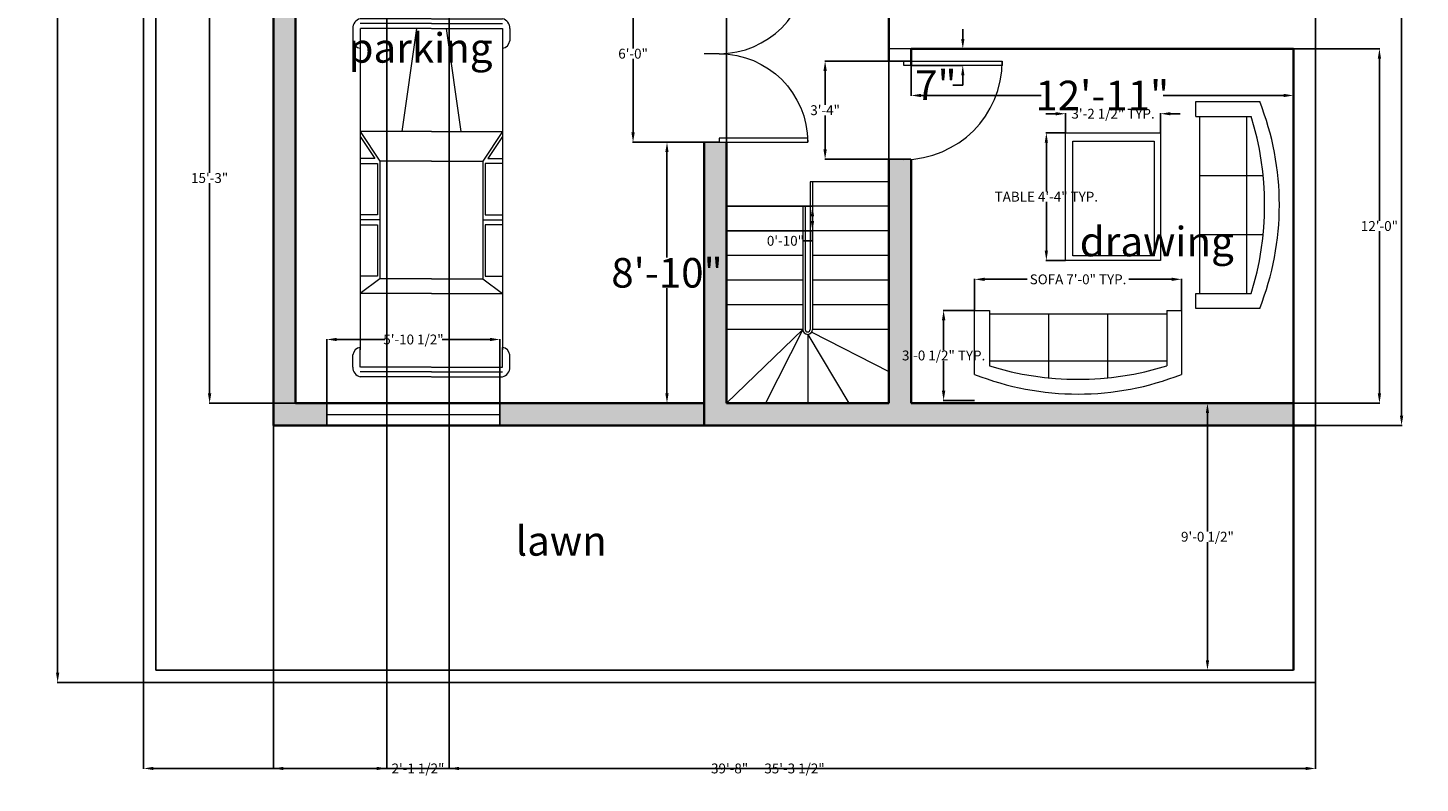
# Model space of a CAD drawing. Units: inches. Extents: x -346 to 220, y 97 to 877.
# Tile 1 of 4: x -346 to 220, y 97 to 404. Entities that reach past the tile are written whole.
import ezdxf

# ---------------------------------------------------------------- set-up
doc = ezdxf.new("R2010")
doc.units = ezdxf.units.IN
doc.header["$MEASUREMENT"] = 0
doc.layers.get('0').update_dxf_attribs({"color": 3})
for name, color, linetype, lineweight in [('A-AREA-IDEN', 130, 'Continuous', 25), ('A-FLOR-STRS', 3, 'Continuous', 18), ('A-FURN', 8, 'Continuous', 18), ('A-WALL', 7, 'Continuous', 35), ('C-PRKG-VEHI', 8, 'Continuous', 13), ('C-PROP', 94, 'Continuous', 25), ('dim', 170, 'Continuous', 13), ('door', 20, 'Continuous', 18)]:
    doc.layers.add(name, color=color, linetype=linetype, lineweight=lineweight)
doc.layers.add('A-WALL-PATT', color=61, linetype='Continuous', lineweight=13, true_color=0xe5e878)
doc.styles.get("Standard").update_dxf_attribs({"font": 'arial.ttf'})
doc.dimstyles.get("Standard").update_dxf_attribs({"dimtxt": 4, "dimasz": 4, "dimexe": 0.18, "dimexo": 0.0625, "dimgap": 0.09, "dimtad": 0, "dimtih": 1, "dimtoh": 1, "dimdec": 0, "dimzin": 0, "dimdsep": 46, "dimlunit": 3, "dimtxsty": 'Standard', "dimcen": 0.09, "dimadec": 0, "dimazin": 0, "dimtfac": 1, "dimtdec": 0, "dimtofl": 0, "dimtmove": 0, "dimatfit": 3, "dimfxl": 1, "dimtolj": 1, "dimtzin": 0, "dimarcsym": 0})

# ---------------------------------------------------------------- blocks, each defined once
blk = doc.blocks.new('*D7')
at = {"layer": 'Defpoints', "color": 0, "transparency": 16777216}
for p in [(-71.23, 357.75), (-86.38, 251.75), (-71.23, 251.75)]:
    blk.add_point(p, dxfattribs=at)
at = {"layer": 'dim', "color": 0, "lineweight": -2, "transparency": 16777216}
for p, q in [((-71.29, 357.75), (-86.56, 357.75)), ((-86.38, 353.75), (-86.38, 310.96)), ((-86.38, 255.75), (-86.38, 298.53)), ((-71.29, 251.75), (-86.56, 251.75))]:
    blk.add_line(p, q, dxfattribs=at)
at = {"layer": 'dim', "color": 0, "transparency": 16777216}
for points in [[(-87.05, 353.75), (-85.72, 353.75), (-86.38, 357.75)], [(-87.05, 255.75), (-85.72, 255.75), (-86.38, 251.75)]]:
    blk.add_solid(points, dxfattribs=at)
at = {"layer": 'dim', "color": 0, "transparency": 16777216, "insert": (-86.38, 304.75), "char_height": 4, "attachment_point": 5}
blk.add_mtext('\\A1;{\\H3x;8\'-10"}', dxfattribs=at)
blk = doc.blocks.new('*D9')
at = {"layer": 'Defpoints', "color": 0, "transparency": 16777216}
for p in [(12.77, 395.75), (168.07, 395.75), (168.07, 376.78)]:
    blk.add_point(p, dxfattribs=at)
at = {"layer": 'dim', "color": 0, "lineweight": -2, "transparency": 16777216}
for p, q in [((12.77, 395.68), (12.77, 376.6)), ((168.07, 395.68), (168.07, 376.6)), ((16.77, 376.78), (65.62, 376.78)), ((164.07, 376.78), (115.22, 376.78))]:
    blk.add_line(p, q, dxfattribs=at)
at = {"layer": 'dim', "color": 0, "transparency": 16777216}
for points in [[(16.77, 377.44), (16.77, 376.11), (12.77, 376.78)], [(164.07, 377.44), (164.07, 376.11), (168.07, 376.78)]]:
    blk.add_solid(points, dxfattribs=at)
at = {"layer": 'dim', "color": 0, "transparency": 16777216, "insert": (90.42, 376.78), "char_height": 4, "attachment_point": 5}
blk.add_mtext('\\A1;{\\H3x;12\'-11"}', dxfattribs=at)
blk = doc.blocks.new('*D10')
at = {"layer": 'Defpoints', "color": 0, "transparency": 16777216}
for p in [(12.77, 395.75), (12.77, 389), (33.77, 389)]:
    blk.add_point(p, dxfattribs=at)
at = {"layer": 'dim', "color": 0, "lineweight": -2, "transparency": 16777216}
for p, q in [((33.77, 399.75), (33.77, 403.75)), ((12.84, 395.75), (33.95, 395.75)), ((12.84, 389), (33.95, 389)), ((33.77, 385), (33.77, 381)), ((33.77, 381), (29.77, 381))]:
    blk.add_line(p, q, dxfattribs=at)
at = {"layer": 'dim', "color": 0, "transparency": 16777216}
for points in [[(33.11, 399.75), (34.44, 399.75), (33.77, 395.75)], [(33.11, 385), (34.44, 385), (33.77, 389)]]:
    blk.add_solid(points, dxfattribs=at)
at = {"layer": 'dim', "color": 0, "transparency": 16777216, "insert": (22.84, 381), "char_height": 4, "attachment_point": 5}
blk.add_mtext('\\A1;{\\H3x;7"}', dxfattribs=at)
blk = doc.blocks.new('*U12')
for p, q in [((0, 0), (0, -6)), ((40, 0), (40, -6))]:
    blk.add_line(p, q)
blk.add_lwpolyline([(0, 0), (0, 40), (1.75, 40), (1.75, 0)], close=True)
blk.add_arc((0, 0), 40, 0, 90)
blk = doc.blocks.new('*U13')
for p, q in [((0, 0), (0, -6)), ((36, 0), (36, -6))]:
    blk.add_line(p, q)
blk.add_lwpolyline([(0, 0), (0, 36), (1.75, 36), (1.75, 0)], close=True)
blk.add_arc((0, 0), 36, 0, 90)
blk = doc.blocks.new('Sofa - Roundback 7 ft.')
for p, q in [((-12.00002, -32.4421), (-12.00003, -6.5971)), ((11.99997, -32.4421), (11.99998, -6.5971)), ((-36.000027, -34), (-36.000027, -11.4696)), ((-35.999844, -13.3819), (35.9998, -13.3819)), ((35.99998, -34), (35.99998, -11.4696)), ((-36.000027, -32.4421), (35.99998, -32.4421))]:
    blk.add_line(p, q)
for points in [[(-36.000027, -34), (-42.000027, -34), (-42.000027, -8)], [(41.99998, -8), (41.99998, -34), (35.99998, -34)]]:
    blk.add_lwpolyline(points)
for centre, radius, start, end in [((0, -114.25), 114.25, 68.43141, 111.5686), ((-0.00001, -127.1968), 121.1968, 72.72033, 107.2797)]:
    blk.add_arc(centre, radius, start, end)
blk = doc.blocks.new('*U27')
for p, q in [((0.1, -0.41), (0.1, 38.35)), ((2.77, -0.41), (2.77, 38.31)), ((5.44, 42.31), (12.12, 42.31)), ((5.44, -0.41), (5.44, 38.24)), ((5.45, 38.31), (16.12, 38.31)), ((16.12, 38.31), (180.34, 38.31)), ((61.52, -0.41), (61.52, 38.31)), ((61.52, 38.31), (77.54, 27.62)), ((64.19, 38.31), (76.2, 30.29)), ((76.2, 30.29), (76.2, 38.31)), ((78.87, 38.31), (78.87, 28.96)), ((106.91, 28.96), (106.91, 38.31)), ((109.58, 27.62), (109.58, 38.31)), ((112.25, 38.31), (112.25, 28.96)), ((140.29, 28.96), (140.29, 38.31)), ((141.62, 27.62), (149.64, 38.31)), ((149.64, -0.41), (149.64, 38.31)), ((189.69, 38.31), (179.01, 38.31)), ((189.69, 42.31), (183.01, 42.31)), ((189.69, -0.41), (189.69, 38.24)), ((192.36, -0.41), (192.36, 38.31)), ((195.03, -0.41), (195.03, 38.35)), ((77.54, 27.62), (141.62, 27.62)), ((77.54, -0.41), (77.54, 27.62)), ((78.87, 28.96), (106.91, 28.96)), ((112.25, 28.96), (140.29, 28.96)), ((141.62, -0.41), (141.62, 27.62)), ((5.44, 7.6), (61.52, 15.61)), ((0.1, -0.42), (0.1, -39.18)), ((2.77, -0.41), (2.77, -39.13)), ((5.44, -0.42), (5.44, -39.07)), ((61.52, -0.41), (61.52, -39.13)), ((77.54, -0.41), (77.54, -28.45)), ((141.62, -0.41), (141.62, -28.45)), ((149.64, -0.41), (149.64, -39.13)), ((189.69, -0.42), (189.69, -39.07)), ((192.36, -0.41), (192.36, -39.13)), ((195.03, -0.42), (195.03, -39.18)), ((5.44, -8.42), (61.52, -16.43)), ((61.52, -39.13), (77.54, -28.45)), ((77.54, -28.45), (141.62, -28.45)), ((78.87, -39.13), (78.87, -29.79)), ((78.87, -29.79), (106.91, -29.79)), ((106.91, -29.79), (106.91, -39.13)), ((109.58, -28.45), (109.58, -39.13)), ((112.25, -29.79), (140.29, -29.79)), ((112.25, -39.13), (112.25, -29.79)), ((140.29, -29.79), (140.29, -39.13)), ((141.62, -28.45), (149.64, -39.13)), ((64.19, -39.13), (76.2, -31.12)), ((76.2, -31.12), (76.2, -39.13)), ((5.44, -43.14), (12.12, -43.14)), ((5.45, -39.13), (16.12, -39.13)), ((16.12, -39.13), (180.34, -39.13)), ((189.69, -39.13), (179.01, -39.13)), ((189.69, -43.14), (183.01, -43.14))]:
    blk.add_line(p, q)
for centre, radius, start, end in [((5.06, 37.26), 5.06, 85.64554, 168.0943), ((11.45, 37.64), 4.72, 8.13011, 81.86996), ((183.68, 37.64), 4.72, 98.13004, 171.8699), ((190.07, 37.26), 5.06, 11.90574, 94.35446), ((5.06, -38.09), 5.06, 191.9057, 274.3545), ((11.45, -38.46), 4.72, 278.13, 351.8699), ((183.68, -38.46), 4.72, 188.1301, 261.87), ((190.07, -38.09), 5.06, 265.6455, 348.0943)]:
    blk.add_arc(centre, radius, start, end)
blk = doc.blocks.new('TABLE-COFFEE-RECT')
for points in [[(0, 51.83), (38.64, 51.83), (38.64, 0), (0, 0)], [(2.97, 48.5), (36.03, 48.5), (36.03, 1.93), (2.97, 1.93)]]:
    blk.add_lwpolyline(points, close=True)
blk = doc.blocks.new('*D32')
at = {"layer": 'Defpoints', "color": 0, "transparency": 16777216}
for p in [(38.59, 302.1), (38.59, 289.5), (122.59, 289.5)]:
    blk.add_point(p, dxfattribs=at)
at = {"layer": 'dim', "color": 0, "lineweight": -2, "transparency": 16777216}
for p, q in [((38.59, 289.56), (38.59, 302.28)), ((42.59, 302.1), (59.94, 302.1)), ((118.59, 302.1), (101.25, 302.1)), ((122.59, 289.56), (122.59, 302.28))]:
    blk.add_line(p, q, dxfattribs=at)
at = {"layer": 'dim', "color": 0, "transparency": 16777216}
for points in [[(42.59, 302.77), (42.59, 301.43), (38.59, 302.1)], [(118.59, 302.77), (118.59, 301.43), (122.59, 302.1)]]:
    blk.add_solid(points, dxfattribs=at)
at = {"layer": 'dim', "color": 0, "transparency": 16777216, "insert": (80.59, 302.1), "char_height": 4, "attachment_point": 5}
blk.add_mtext('\\A1;SOFA 7\'-0" TYP.', dxfattribs=at)
blk = doc.blocks.new('*D33')
at = {"layer": 'Defpoints', "color": 0, "transparency": 16777216}
for p in [(38.59, 289.5), (25.99, 252.83), (38.59, 252.83)]:
    blk.add_point(p, dxfattribs=at)
at = {"layer": 'dim', "color": 0, "lineweight": -2, "transparency": 16777216}
for p, q in [((38.53, 289.5), (25.81, 289.5)), ((25.99, 285.5), (25.99, 273.33)), ((25.99, 256.83), (25.99, 269.01)), ((38.53, 252.83), (25.81, 252.83))]:
    blk.add_line(p, q, dxfattribs=at)
at = {"layer": 'dim', "color": 0, "transparency": 16777216}
for points in [[(25.32, 285.5), (26.66, 285.5), (25.99, 289.5)], [(25.32, 256.83), (26.66, 256.83), (25.99, 252.83)]]:
    blk.add_solid(points, dxfattribs=at)
at = {"layer": 'dim', "color": 0, "transparency": 16777216, "insert": (25.99, 271.17), "char_height": 4, "attachment_point": 5}
blk.add_mtext('\\A1;3\'-0 1/2" TYP.', dxfattribs=at)
blk = doc.blocks.new('*D42')
at = {"layer": 'Defpoints', "color": 0, "transparency": 16777216}
for p in [(67.71, 361.58), (75.48, 361.58), (75.48, 309.76)]:
    blk.add_point(p, dxfattribs=at)
at = {"layer": 'dim', "color": 0, "lineweight": -2, "transparency": 16777216}
for p, q in [((75.42, 361.58), (67.53, 361.58)), ((67.71, 357.58), (67.71, 337.76)), ((67.71, 313.76), (67.71, 333.58)), ((75.42, 309.76), (67.53, 309.76))]:
    blk.add_line(p, q, dxfattribs=at)
at = {"layer": 'dim', "color": 0, "transparency": 16777216}
for points in [[(67.04, 357.58), (68.37, 357.58), (67.71, 361.58)], [(67.04, 313.76), (68.37, 313.76), (67.71, 309.76)]]:
    blk.add_solid(points, dxfattribs=at)
at = {"layer": 'dim', "color": 0, "transparency": 16777216, "insert": (67.71, 335.67), "char_height": 4, "attachment_point": 5}
blk.add_mtext('\\A1;TABLE 4\'-4" TYP.', dxfattribs=at)
blk = doc.blocks.new('*D43')
at = {"layer": 'Defpoints', "color": 0, "transparency": 16777216}
for p in [(114.12, 369.36), (75.48, 361.58), (114.12, 361.58)]:
    blk.add_point(p, dxfattribs=at)
at = {"layer": 'dim', "color": 0, "lineweight": -2, "transparency": 16777216}
for p, q in [((71.48, 369.36), (67.48, 369.36)), ((75.48, 361.64), (75.48, 369.54)), ((114.12, 361.64), (114.12, 369.54)), ((118.12, 369.36), (122.12, 369.36))]:
    blk.add_line(p, q, dxfattribs=at)
at = {"layer": 'dim', "color": 0, "transparency": 16777216}
for points in [[(71.48, 370.02), (71.48, 368.69), (75.48, 369.36)], [(118.12, 370.02), (118.12, 368.69), (114.12, 369.36)]]:
    blk.add_solid(points, dxfattribs=at)
at = {"layer": 'dim', "color": 0, "transparency": 16777216, "insert": (94.8, 369.36), "char_height": 4, "attachment_point": 5}
blk.add_mtext('\\A1;3\'-2 1/2" TYP.', dxfattribs=at)
blk = doc.blocks.new('*D48')
at = {"layer": 'Defpoints', "color": 0, "transparency": 16777216}
for p in [(-298.95, 138.35), (177.07, 138.35), (177.07, 103.43)]:
    blk.add_point(p, dxfattribs=at)
at = {"layer": 'dim', "color": 0, "lineweight": -2, "transparency": 16777216}
for p, q in [((-298.95, 138.29), (-298.95, 103.25)), ((177.07, 138.29), (177.07, 103.25)), ((-294.95, 103.43), (-67.9, 103.43)), ((173.07, 103.43), (-53.98, 103.43))]:
    blk.add_line(p, q, dxfattribs=at)
at = {"layer": 'dim', "color": 0, "transparency": 16777216}
for points in [[(-294.95, 104.09), (-294.95, 102.76), (-298.95, 103.43)], [(173.07, 104.09), (173.07, 102.76), (177.07, 103.43)]]:
    blk.add_solid(points, dxfattribs=at)
at = {"layer": 'dim', "color": 0, "transparency": 16777216, "insert": (-60.94, 103.43), "char_height": 4, "attachment_point": 5}
blk.add_mtext('\\A1;39\'-8"', dxfattribs=at)
blk = doc.blocks.new('*D49')
at = {"layer": 'Defpoints', "color": 0, "transparency": 16777216}
for p in [(-333.87, 835.75), (-298.95, 835.75), (-298.95, 138.35)]:
    blk.add_point(p, dxfattribs=at)
at = {"layer": 'dim', "color": 0, "lineweight": -2, "transparency": 16777216}
for p, q in [((-299.01, 835.75), (-334.05, 835.75)), ((-333.87, 831.75), (-333.87, 489.21)), ((-333.87, 142.35), (-333.87, 484.89)), ((-299.01, 138.35), (-334.05, 138.35))]:
    blk.add_line(p, q, dxfattribs=at)
at = {"layer": 'dim', "color": 0, "transparency": 16777216}
for points in [[(-334.54, 831.75), (-333.21, 831.75), (-333.87, 835.75)], [(-334.54, 142.35), (-333.21, 142.35), (-333.87, 138.35)]]:
    blk.add_solid(points, dxfattribs=at)
at = {"layer": 'dim', "color": 0, "transparency": 16777216, "insert": (-333.87, 487.05), "char_height": 4, "attachment_point": 5}
blk.add_mtext('\\A1;58\'-1 1/2"', dxfattribs=at)
blk = doc.blocks.new('*D50')
at = {"layer": 'Defpoints', "color": 0, "transparency": 16777216}
for p in [(-246.23, 242.75), (177.07, 242.75), (177.07, 103.43)]:
    blk.add_point(p, dxfattribs=at)
at = {"layer": 'dim', "color": 0, "lineweight": -2, "transparency": 16777216}
for p, q in [((-246.23, 242.68), (-246.23, 103.25)), ((177.07, 242.68), (177.07, 103.25)), ((-242.23, 103.43), (-46.2, 103.43)), ((173.07, 103.43), (-22.96, 103.43))]:
    blk.add_line(p, q, dxfattribs=at)
at = {"layer": 'dim', "color": 0, "transparency": 16777216}
for points in [[(-242.23, 104.09), (-242.23, 102.76), (-246.23, 103.43)], [(173.07, 104.09), (173.07, 102.76), (177.07, 103.43)]]:
    blk.add_solid(points, dxfattribs=at)
at = {"layer": 'dim', "color": 0, "transparency": 16777216, "insert": (-34.58, 103.43), "char_height": 4, "attachment_point": 5}
blk.add_mtext('\\A1;35\'-3 1/2"', dxfattribs=at)
blk = doc.blocks.new('*D51')
at = {"layer": 'Defpoints', "color": 0, "transparency": 16777216}
for p in [(177.07, 835.75), (212, 835.75), (177.07, 242.75)]:
    blk.add_point(p, dxfattribs=at)
at = {"layer": 'dim', "color": 0, "lineweight": -2, "transparency": 16777216}
for p, q in [((177.13, 835.75), (212.18, 835.75)), ((212, 831.75), (212, 541.38)), ((212, 246.75), (212, 537.11)), ((177.13, 242.75), (212.18, 242.75))]:
    blk.add_line(p, q, dxfattribs=at)
at = {"layer": 'dim', "color": 0, "transparency": 16777216}
for points in [[(211.33, 831.75), (212.66, 831.75), (212, 835.75)], [(211.33, 246.75), (212.66, 246.75), (212, 242.75)]]:
    blk.add_solid(points, dxfattribs=at)
at = {"layer": 'dim', "color": 0, "transparency": 16777216, "insert": (212, 539.25), "char_height": 4, "attachment_point": 5}
blk.add_mtext('\\A1;49\'-5"', dxfattribs=at)
blk = doc.blocks.new('*D52')
at = {"layer": 'Defpoints', "color": 0, "transparency": 16777216}
for p in [(-246.23, 870.67), (-246.23, 242.75), (-293.95, 143.35)]:
    blk.add_point(p, dxfattribs=at)
at = {"layer": 'dim', "color": 0, "lineweight": -2, "transparency": 16777216}
for p, q in [((-293.95, 143.41), (-293.95, 870.85)), ((-289.95, 870.67), (-281.71, 870.67)), ((-250.23, 870.67), (-258.47, 870.67)), ((-246.23, 242.81), (-246.23, 870.85))]:
    blk.add_line(p, q, dxfattribs=at)
at = {"layer": 'dim', "color": 0, "transparency": 16777216}
for points in [[(-289.95, 871.34), (-289.95, 870), (-293.95, 870.67)], [(-250.23, 871.34), (-250.23, 870), (-246.23, 870.67)]]:
    blk.add_solid(points, dxfattribs=at)
at = {"layer": 'dim', "color": 0, "transparency": 16777216, "insert": (-270.09, 870.67), "char_height": 4, "attachment_point": 5}
blk.add_mtext('\\A1;3\'-11 1/2"', dxfattribs=at)
blk = doc.blocks.new('*D53')
at = {"layer": 'Defpoints', "color": 0, "transparency": 16777216}
for p in [(133.15, 251.75), (168.07, 251.75), (168.07, 143.35)]:
    blk.add_point(p, dxfattribs=at)
at = {"layer": 'dim', "color": 0, "lineweight": -2, "transparency": 16777216}
for p, q in [((168.01, 251.75), (132.97, 251.75)), ((133.15, 247.75), (133.15, 199.71)), ((133.15, 147.35), (133.15, 195.39)), ((168.01, 143.35), (132.97, 143.35))]:
    blk.add_line(p, q, dxfattribs=at)
at = {"layer": 'dim', "color": 0, "transparency": 16777216}
for points in [[(132.48, 247.75), (133.81, 247.75), (133.15, 251.75)], [(132.48, 147.35), (133.81, 147.35), (133.15, 143.35)]]:
    blk.add_solid(points, dxfattribs=at)
at = {"layer": 'dim', "color": 0, "transparency": 16777216, "insert": (133.15, 197.55), "char_height": 4, "attachment_point": 5}
blk.add_mtext('\\A1;9\'-0 1/2"', dxfattribs=at)
blk = doc.blocks.new('*D57')
at = {"layer": 'Defpoints', "color": 0, "transparency": 16777216}
for p in [(168.07, 395.75), (168.07, 251.75), (203, 251.75)]:
    blk.add_point(p, dxfattribs=at)
at = {"layer": 'dim', "color": 0, "lineweight": -2, "transparency": 16777216}
for p, q in [((168.13, 395.75), (203.18, 395.75)), ((203, 391.75), (203, 325.88)), ((203, 255.75), (203, 321.61)), ((168.13, 251.75), (203.18, 251.75))]:
    blk.add_line(p, q, dxfattribs=at)
at = {"layer": 'dim', "color": 0, "transparency": 16777216}
for points in [[(202.33, 391.75), (203.66, 391.75), (203, 395.75)], [(202.33, 255.75), (203.66, 255.75), (203, 251.75)]]:
    blk.add_solid(points, dxfattribs=at)
at = {"layer": 'dim', "color": 0, "transparency": 16777216, "insert": (203, 323.75), "char_height": 4, "attachment_point": 5}
blk.add_mtext('\\A1;12\'-0"', dxfattribs=at)
blk = doc.blocks.new('*D58')
at = {"layer": 'Defpoints', "color": 0, "transparency": 16777216}
for p in [(3.77, 870.67), (3.77, 341.75), (-62.23, 331.75)]:
    blk.add_point(p, dxfattribs=at)
at = {"layer": 'dim', "color": 0, "lineweight": -2, "transparency": 16777216}
for p, q in [((-62.23, 331.81), (-62.23, 870.85)), ((-58.23, 870.67), (-34.63, 870.67)), ((-0.23, 870.67), (-23.82, 870.67)), ((3.77, 341.81), (3.77, 870.85))]:
    blk.add_line(p, q, dxfattribs=at)
at = {"layer": 'dim', "color": 0, "transparency": 16777216}
for points in [[(-58.23, 871.34), (-58.23, 870), (-62.23, 870.67)], [(-0.23, 871.34), (-0.23, 870), (3.77, 870.67)]]:
    blk.add_solid(points, dxfattribs=at)
at = {"layer": 'dim', "color": 0, "transparency": 16777216, "insert": (-29.23, 870.67), "char_height": 4, "attachment_point": 5}
blk.add_mtext('\\A1;5\'-6"', dxfattribs=at)
blk = doc.blocks.new('*D59')
at = {"layer": 'Defpoints', "color": 0, "transparency": 16777216}
for p in [(-272.15, 434.75), (-237.23, 434.75), (-237.23, 251.75)]:
    blk.add_point(p, dxfattribs=at)
at = {"layer": 'dim', "color": 0, "lineweight": -2, "transparency": 16777216}
for p, q in [((-237.29, 434.75), (-272.33, 434.75)), ((-272.15, 430.75), (-272.15, 345.38)), ((-272.15, 255.75), (-272.15, 341.11)), ((-237.29, 251.75), (-272.33, 251.75))]:
    blk.add_line(p, q, dxfattribs=at)
at = {"layer": 'dim', "color": 0, "transparency": 16777216}
for points in [[(-272.82, 430.75), (-271.48, 430.75), (-272.15, 434.75)], [(-272.82, 255.75), (-271.48, 255.75), (-272.15, 251.75)]]:
    blk.add_solid(points, dxfattribs=at)
at = {"layer": 'dim', "color": 0, "transparency": 16777216, "insert": (-272.15, 343.25), "char_height": 4, "attachment_point": 5}
blk.add_mtext('\\A1;15\'-3"', dxfattribs=at)
blk = doc.blocks.new('*D61')
at = {"layer": 'Defpoints', "color": 0, "transparency": 16777216}
for p in [(-100.15, 429.75), (-65.23, 429.75), (-65.23, 357.75)]:
    blk.add_point(p, dxfattribs=at)
at = {"layer": 'dim', "color": 0, "lineweight": -2, "transparency": 16777216}
for p, q in [((-65.29, 429.75), (-100.33, 429.75)), ((-100.15, 425.75), (-100.15, 395.88)), ((-100.15, 361.75), (-100.15, 391.61)), ((-65.29, 357.75), (-100.33, 357.75))]:
    blk.add_line(p, q, dxfattribs=at)
at = {"layer": 'dim', "color": 0, "transparency": 16777216}
for points in [[(-100.82, 425.75), (-99.48, 425.75), (-100.15, 429.75)], [(-100.82, 361.75), (-99.48, 361.75), (-100.15, 357.75)]]:
    blk.add_solid(points, dxfattribs=at)
at = {"layer": 'dim', "color": 0, "transparency": 16777216, "insert": (-100.15, 393.75), "char_height": 4, "attachment_point": 5}
blk.add_mtext('\\A1;6\'-0"', dxfattribs=at)
blk = doc.blocks.new('*D66')
at = {"layer": 'Defpoints', "color": 0, "transparency": 16777216}
for p in [(-22.15, 390.75), (12.77, 390.75), (12.77, 350.86)]:
    blk.add_point(p, dxfattribs=at)
at = {"layer": 'dim', "color": 0, "lineweight": -2, "transparency": 16777216}
for p, q in [((12.71, 390.75), (-22.33, 390.75)), ((-22.15, 386.75), (-22.15, 372.94)), ((-22.15, 354.86), (-22.15, 368.67)), ((12.71, 350.86), (-22.33, 350.86))]:
    blk.add_line(p, q, dxfattribs=at)
at = {"layer": 'dim', "color": 0, "transparency": 16777216}
for points in [[(-22.82, 386.75), (-21.48, 386.75), (-22.15, 390.75)], [(-22.82, 354.86), (-21.48, 354.86), (-22.15, 350.86)]]:
    blk.add_solid(points, dxfattribs=at)
at = {"layer": 'dim', "color": 0, "transparency": 16777216, "insert": (-22.15, 370.8), "char_height": 4, "attachment_point": 5}
blk.add_mtext('\\A1;3\'-4"', dxfattribs=at)
blk = doc.blocks.new('*D68')
at = {"layer": 'Defpoints', "color": 0, "transparency": 16777216}
for p in [(-154.23, 277.67), (-224.48, 242.75), (-154.23, 242.75)]:
    blk.add_point(p, dxfattribs=at)
at = {"layer": 'dim', "color": 0, "lineweight": -2, "transparency": 16777216}
for p, q in [((-224.48, 242.81), (-224.48, 277.85)), ((-220.48, 277.67), (-200.98, 277.67)), ((-158.23, 277.67), (-177.73, 277.67)), ((-154.23, 242.81), (-154.23, 277.85))]:
    blk.add_line(p, q, dxfattribs=at)
at = {"layer": 'dim', "color": 0, "transparency": 16777216}
for points in [[(-220.48, 278.34), (-220.48, 277), (-224.48, 277.67)], [(-158.23, 278.34), (-158.23, 277), (-154.23, 277.67)]]:
    blk.add_solid(points, dxfattribs=at)
at = {"layer": 'dim', "color": 0, "transparency": 16777216, "insert": (-189.36, 277.67), "char_height": 4, "attachment_point": 5}
blk.add_mtext('\\A1;5\'-10 1/2"', dxfattribs=at)
blk = doc.blocks.new('*D71')
at = {"layer": 'Defpoints', "color": 0, "transparency": 16777216}
for p in [(-174.82, 474.69), (-200.23, 443.75), (-174.82, 103.43)]:
    blk.add_point(p, dxfattribs=at)
at = {"layer": 'dim', "color": 0, "lineweight": -2, "transparency": 16777216}
for p, q in [((-174.82, 474.63), (-174.82, 103.25)), ((-200.23, 443.68), (-200.23, 103.25)), ((-204.23, 103.43), (-208.23, 103.43)), ((-170.82, 103.43), (-166.82, 103.43))]:
    blk.add_line(p, q, dxfattribs=at)
at = {"layer": 'dim', "color": 0, "transparency": 16777216}
for points in [[(-204.23, 104.09), (-204.23, 102.76), (-200.23, 103.43)], [(-170.82, 104.09), (-170.82, 102.76), (-174.82, 103.43)]]:
    blk.add_solid(points, dxfattribs=at)
at = {"layer": 'dim', "color": 0, "transparency": 16777216, "insert": (-187.52, 103.43), "char_height": 4, "attachment_point": 5}
blk.add_mtext('\\A1;2\'-1 1/2"', dxfattribs=at)
blk = doc.blocks.new('*D73')
at = {"layer": 'Defpoints', "color": 0, "transparency": 16777216}
for p in [(-62.23, 331.75), (-62.23, 321.75), (-27.3, 321.75)]:
    blk.add_point(p, dxfattribs=at)
at = {"layer": 'dim', "color": 0, "lineweight": -2, "transparency": 16777216}
for p, q in [((-62.16, 331.75), (-27.12, 331.75)), ((-27.3, 327.75), (-27.3, 325.75)), ((-62.16, 321.75), (-27.12, 321.75)), ((-27.3, 317.75), (-31.3, 317.75)), ((-27.3, 321.75), (-27.3, 317.75))]:
    blk.add_line(p, q, dxfattribs=at)
at = {"layer": 'dim', "color": 0, "transparency": 16777216}
for points in [[(-27.97, 327.75), (-26.63, 327.75), (-27.3, 331.75)], [(-27.97, 325.75), (-26.63, 325.75), (-27.3, 321.75)]]:
    blk.add_solid(points, dxfattribs=at)
at = {"layer": 'dim', "color": 0, "transparency": 16777216, "insert": (-38.26, 317.75), "char_height": 4, "attachment_point": 5}
blk.add_mtext('\\A1;0\'-10"', dxfattribs=at)

msp = doc.modelspace()

# ---------------------------------------------------------------- hatches: boundary and pattern name
at = {"layer": 'A-WALL-PATT'}
h = msp.add_hatch(color=256, dxfattribs=at)
h.dxf.hatch_style = 1
h.paths.add_polyline_path([(168.07, 251.75), (33.77, 251.75), (12.77, 251.75), (12.77, 350.86, -0.01877), (9.77, 350.75), (3.77, 350.75), (3.77, 251.75), (-62.23, 251.75), (-62.23, 357.75), (-65.23, 357.75), (-71.23, 357.75), (-71.23, 242.75), (168.07, 242.75)])
h.paths.add_polyline_path([(-71.23, 251.75), (-154.23, 251.75), (-154.23, 242.75), (-71.23, 242.75)])
h.paths.add_polyline_path([(-224.48, 251.75), (-237.23, 251.75), (-237.23, 434.75), (-184.39, 434.75), (-184.39, 443.75), (-200.23, 443.75), (-200.23, 449.16), (-209.23, 449.16), (-209.23, 443.75), (-246.23, 443.75), (-246.23, 242.75), (-224.48, 242.75)])

# ---------------------------------------------------------------- linework, layer by layer
at = {"layer": 'A-FLOR-STRS'}
for p, q in [((-28.23, 341.75), (-28.23, 281.75)), ((3.77, 341.75), (-28.23, 341.75)), ((-27.23, 341.75), (-27.23, 281.75)), ((-30.23, 331.75), (-62.23, 331.75)), ((-31.23, 331.75), (-31.23, 281.75)), ((-30.23, 331.75), (-30.23, 281.75)), ((3.77, 331.75), (-27.23, 331.75)), ((-31.23, 321.75), (-62.23, 321.75)), ((3.77, 321.75), (-27.23, 321.75)), ((-31.23, 311.75), (-62.23, 311.75)), ((3.77, 311.75), (-27.23, 311.75)), ((-31.23, 301.75), (-62.23, 301.75)), ((-31.23, 301.75), (-62.23, 301.75)), ((3.77, 301.75), (-27.23, 301.75)), ((-31.23, 291.75), (-62.23, 291.75)), ((3.77, 291.75), (-27.23, 291.75)), ((-31.23, 281.75), (-62.23, 281.75)), ((-31.23, 281.75), (-62.23, 251.75)), ((-31.23, 281.75), (-46.34, 251.75)), ((-29.23, 279.75), (-29.23, 251.75)), ((-29.23, 279.75), (-12.57, 251.75)), ((-27.56, 280.64), (3.77, 264.72)), ((3.77, 281.75), (-27.23, 281.75))]:
    msp.add_line(p, q, dxfattribs=at)
for radius in [2, 1]:
    msp.add_arc((-29.23, 281.75), radius, 180, 0, dxfattribs=at)
at = {"layer": 'A-WALL'}
for p, q in [((-246.23, 443.75), (-246.23, 242.75)), ((-237.23, 434.75), (-237.23, 251.75)), ((3.77, 434.75), (3.77, 390.75)), ((3.77, 434.75), (3.77, 390.75)), ((-62.23, 393.62), (-62.23, 393.87)), ((-62.23, 393.62), (-62.23, 393.87)), ((168.07, 395.75), (12.77, 395.75)), ((12.77, 395.75), (12.77, 389)), ((12.77, 395.75), (12.77, 389)), ((168.07, 143.35), (168.07, 395.75)), ((-71.23, 251.75), (-71.23, 357.75)), ((-71.23, 242.75), (-71.23, 357.75)), ((-62.23, 251.75), (-62.23, 357.75)), ((-62.23, 251.75), (-62.23, 357.75)), ((3.77, 350.75), (3.77, 251.75)), ((3.77, 350.75), (3.77, 251.75)), ((12.77, 350.86), (12.77, 251.75)), ((12.77, 350.86), (12.77, 251.75)), ((-237.23, 251.75), (-71.23, 251.75)), ((3.77, 251.75), (-62.23, 251.75)), ((33.77, 251.75), (12.77, 251.75)), ((33.77, 251.75), (168.07, 251.75)), ((-246.23, 242.75), (177.07, 242.75))]:
    msp.add_line(p, q, dxfattribs=at)
at = {"layer": 'C-PROP'}
for p, q in [((-298.95, 138.35), (-298.95, 835.75)), ((-293.95, 143.35), (-293.95, 830.75)), ((177.07, 138.35), (177.07, 644.75)), ((-293.95, 143.35), (168.07, 143.35)), ((-298.95, 138.35), (177.07, 138.35))]:
    msp.add_line(p, q, dxfattribs=at)
at = {"layer": 'door'}
for p, q in [((12.77, 395.75), (3.77, 395.75)), ((12.77, 390.75), (3.77, 390.75)), ((-224.48, 251.75), (-224.48, 242.75)), ((-154.23, 251.75), (-154.23, 242.75)), ((-224.48, 247.25), (-154.23, 247.25))]:
    msp.add_line(p, q, dxfattribs=at)

# ---------------------------------------------------------------- block references
at = {"layer": 'A-FURN'}
for p, rotation in [((162.36, 332.3), 270), ((80.59, 255.5), 180)]:
    msp.add_blockref('Sofa - Roundback 7 ft.', p, dxfattribs=dict(at, rotation=rotation))
msp.add_blockref('TABLE-COFFEE-RECT', (75.48, 309.76), dxfattribs=at)
at = {"layer": 'C-PRKG-VEHI', "xscale": 0.7461287105312193, "yscale": 0.7461287105312193, "zscale": 0.7461287105312193, "rotation": 270}
msp.add_blockref('*U27', (-181.78, 408.01), dxfattribs=at)
at = {"layer": 'door', "rotation": 270}
for name, p in [('*U13', (-65.23, 429.75)), ('*U12', (9.77, 390.75))]:
    msp.add_blockref(name, p, dxfattribs=at)
at = {"layer": 'door', "xscale": -1, "rotation": 270}
msp.add_blockref('*U13', (-65.23, 357.75), dxfattribs=at)

# ---------------------------------------------------------------- texts
at = {"layer": 'A-AREA-IDEN', "char_height": 12, "attachment_point": 1}
for s, width, insert in [('parking', 62.6765, (-215.73, 402.09)), ('drawing', 62.6765, (81.28, 323.44)), (' lawn', 179.6897, (-151.5, 201.85))]:
    msp.add_mtext_dynamic_manual_height_columns(s, width=width, gutter_width=1, heights=[0], dxfattribs=dict(at, insert=insert))

# ---------------------------------------------------------------- dimensions: what is measured, and where the dimension line sits
at = {"layer": 'dim'}
for base, p1, p2, picture, middle in [((-246.23, 870.67), (-293.95, 143.35), (-246.23, 242.75), '*D52', (-270.09, 870.67)), ((3.77, 870.67), (-62.23, 331.75), (3.77, 341.75), '*D58', (-29.23, 870.67)), ((-174.82, 103.43), (-200.23, 443.75), (-174.82, 474.69), '*D71', (-187.52, 103.43)), ((-154.2262, 277.6701), (-224.4849, 242.7451), (-154.2262, 242.7451), '*D68', (-189.3556, 277.6701)), ((177.07, 103.43), (-246.23, 242.75), (177.07, 242.75), '*D50', (-34.58, 103.43)), ((177.07, 103.43), (-298.95, 138.35), (177.07, 138.35), '*D48', (-60.94, 103.43))]:
    dim = msp.add_linear_dim(base=base, p1=p1, p2=p2, dimstyle='Standard', override={"dimdec": 1, "dimlfac": 1, "dimrnd": 0, "dimzin": 1, "dimdsep": 46, "dimlunit": 4, "dimfrac": 2}, dxfattribs=at)
    dim.commit()
    dim.dimension.update_dxf_attribs({"geometry": picture, "text_midpoint": middle})
for base, p1, p2, angle, picture, middle in [((-333.87, 835.75), (-298.95, 138.35), (-298.95, 835.75), 90, '*D49', (-333.87, 487.05)), ((212, 835.75), (177.07, 242.75), (177.07, 835.75), 90, '*D51', (212, 539.25)), ((-272.15, 434.75), (-237.23, 251.75), (-237.23, 434.75), 90, '*D59', (-272.15, 343.25)), ((-100.15, 429.75), (-65.23, 357.75), (-65.23, 429.75), 90, '*D61', (-100.15, 393.75)), ((-22.15, 390.75), (12.77, 350.86), (12.77, 390.75), 90, '*D66', (-22.15, 370.8)), ((203, 251.75), (168.07, 395.75), (168.07, 251.75), 270, '*D57', (203, 323.75)), ((-27.3, 321.75), (-62.23, 331.75), (-62.23, 321.75), 270, '*D73', (-38.26, 317.75)), ((133.15, 251.75), (168.07, 143.35), (168.07, 251.75), 90, '*D53', (133.15, 197.55))]:
    dim = msp.add_linear_dim(base=base, p1=p1, p2=p2, angle=angle, dimstyle='Standard', override={"dimdec": 1, "dimlfac": 1, "dimrnd": 0, "dimzin": 1, "dimdsep": 46, "dimlunit": 4, "dimfrac": 2}, dxfattribs=at)
    dim.commit()
    dim.dimension.update_dxf_attribs({"geometry": picture, "text_midpoint": middle})
for base, p1, p2, angle, text, override, picture, middle in [((33.77, 389), (12.77, 395.75), (12.77, 389), 90, '{\\H3x;<>}', {"dimclrd": 0, "dimclre": 0, "dimclrt": 0}, '*D10', (22.84, 381)), ((-86.38, 251.75), (-71.23, 357.75), (-71.23, 251.75), 90, '{\\H3x;<>}', {"dimclrd": 0, "dimclre": 0, "dimclrt": 0}, '*D7', (-86.38, 304.75)), ((67.71, 361.58), (75.48, 309.76), (75.48, 361.58), 90, 'TABLE <> TYP.', {"dimdec": 1, "dimlfac": 1, "dimrnd": 0, "dimzin": 1, "dimdsep": 46, "dimlunit": 4, "dimfrac": 2}, '*D42', (67.71, 335.67)), ((38.59, 302.1), (122.59, 289.5), (38.59, 289.5), 180, 'SOFA <> TYP.', {"dimdec": 1, "dimlfac": 1, "dimrnd": 0, "dimzin": 1, "dimdsep": 46, "dimlunit": 4, "dimfrac": 2}, '*D32', (80.59, 302.1)), ((25.99, 252.83), (38.59, 289.5), (38.59, 252.83), 270, '<> TYP.', {"dimdec": 1, "dimlfac": 1, "dimrnd": 0, "dimzin": 1, "dimdsep": 46, "dimlunit": 4, "dimfrac": 2}, '*D33', (25.99, 271.17))]:
    dim = msp.add_linear_dim(base=base, p1=p1, p2=p2, angle=angle, text=text, dimstyle='Standard', override=override, dxfattribs=at)
    dim.commit()
    dim.dimension.update_dxf_attribs({"geometry": picture, "text_midpoint": middle})
for base, p1, p2, text, override, picture, middle in [((168.07, 376.78), (12.77, 395.75), (168.07, 395.75), '{\\H3x;<>}', {"dimclrd": 0, "dimclre": 0, "dimclrt": 0}, '*D9', (90.42, 376.78)), ((114.12, 369.36), (75.48, 361.58), (114.12, 361.58), '<> TYP.', {"dimdec": 1, "dimlfac": 1, "dimrnd": 0, "dimzin": 1, "dimdsep": 46, "dimlunit": 4, "dimfrac": 2}, '*D43', (94.8, 369.36))]:
    dim = msp.add_linear_dim(base=base, p1=p1, p2=p2, text=text, dimstyle='Standard', override=override, dxfattribs=at)
    dim.commit()
    dim.dimension.update_dxf_attribs({"geometry": picture, "text_midpoint": middle})

doc.saveas('drawing.dxf')
